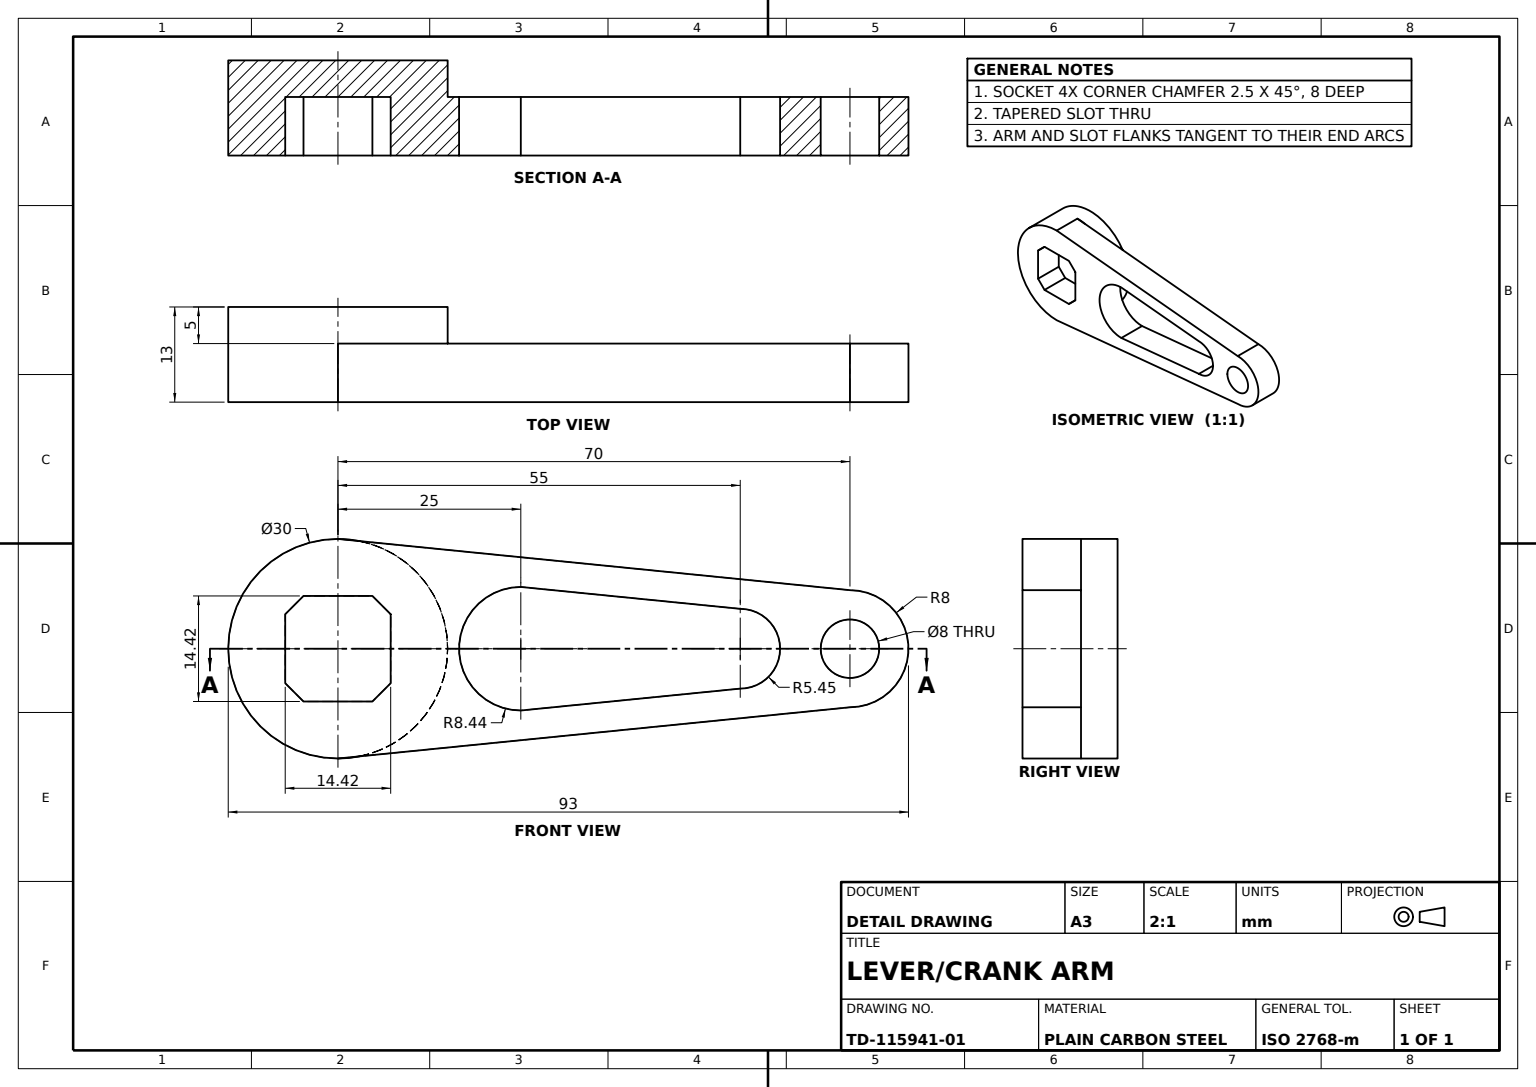
SolidWorks part; units mm, degrees
material "Plain Carbon Steel"
ref_plane "Front Plane" through (0, 0, 0) normal (0, 0, 1) x (1, 0, 0)
ref_plane "Top Plane" through (0, 0, 0) normal (0, 1, 0) x (1, 0, 0)
ref_plane "Right Plane" through (0, 0, 0) normal (1, 0, 0) x (0, 0, -1)
sketch "Lever Profile Sketch" plane through (0, 0, 0) normal (0, 0, 1) x (1, 0, 0)
  line L1 (0, 15) -> (70, 8)
  line L2 (0, -15) -> (70, -8)
  arc A0 (70, -8) -> (70, 8) centre (70, 0) ccw
  arc A1 (0, 15) -> (0, -15) centre (0, 0) ccw
  dimension "D1" = 16
  dimension "D2" = 30
  dimension "D3" = 8
  dimension "D4" = 15
  dimension "D5" = 70
extrude "Lever Arm Plate" add sketch "Lever Profile Sketch" along normal blind 8
sketch "Tapered Slot Sketch" plane through (0, 0, 8) normal (0, 0, 1) x (1, 0, 0)
  line L6 (25, 8.44) -> (55, 5.45)
  line L7 (25, -8.44) -> (55, -5.45)
  arc A2 (55, -5.45) -> (55, 5.45) centre (55, 0) ccw
  arc A3 (25, 8.44) -> (25, -8.44) centre (25, 0) ccw
  dimension "D1" = 5.45
  dimension "D2" = 8.44
  dimension "D3" = 25
  dimension "D4" = 55
  dimension "D5" = 15
extrude "Tapered Slot Cut" cut sketch "Tapered Slot Sketch" against normal blind 8
sketch "Hub Boss Sketch" plane through (0, 0, 0) normal (0, 0, -1) x (-1, 0, 0)
  circle A0 centre (0, 0) radius 15
  dimension "D1" = 30
extrude "Hub Boss" add sketch "Hub Boss Sketch" along normal blind 5
sketch "Pin Hole Sketch" plane through (0, 0, 8) normal (0, 0, 1) x (1, 0, 0)
  circle A0 centre (70, 0) radius 4
  dimension "D1" = 8
extrude "Pin Hole" cut sketch "Pin Hole Sketch" against normal blind 8
sketch "Hex Socket Sketch" plane through (0, 0, 8) normal (0, 0, 1) x (1, 0, 0)
  line L1 (0, 7.21) -> (-4.71, 7.21)
  line L2 (-7.21, 4.71) -> (-7.21, -4.71)
  line L3 (-4.71, -7.21) -> (4.71, -7.21)
  line L4 (7.21, -4.71) -> (7.21, 4.71)
  line L5 (4.71, 7.21) -> (0, 7.21)
  line L7 (7.21, 4.71) -> (4.71, 7.21)
  line L10 (-7.21, 4.71) -> (-4.71, 7.21)
  line L13 (4.71, -7.21) -> (7.21, -4.71)
  line L16 (-4.71, -7.21) -> (-7.21, -4.71)
  dimension "D1" = 17.79
  dimension "D2" = 20.29
  dimension "D3" = 25
  dimension "D4" = 1.23
  dimension "D5" = 3.73
extrude "Hex Socket Cut" cut sketch "Hex Socket Sketch" against normal blind 8
